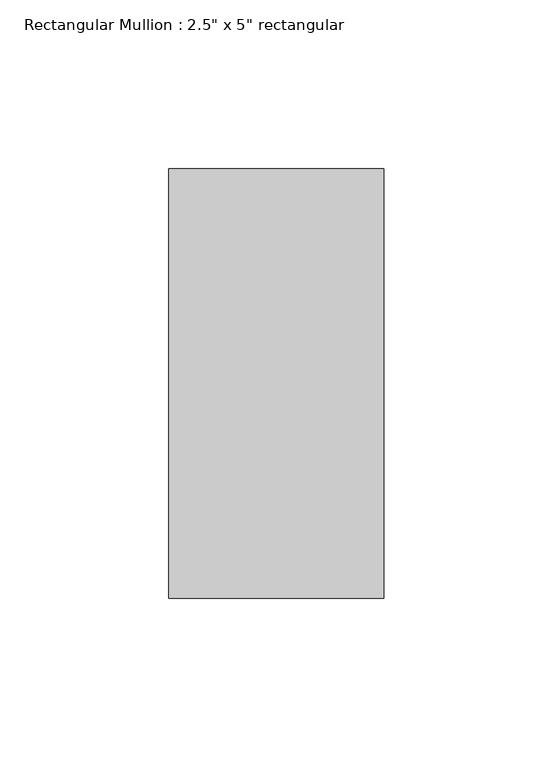
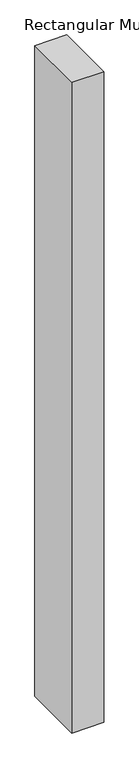
"""IFC4 building model written with IfcOpenShell, lengths in millimetres: member geometry."""

from ifc_helpers import new_model, si_unit, frame, origin, place, context, project, spatial, polyline, outline, extrude, source, transform, mapped, element, save


def member_80f955c2(model_context):
    return source(origin(), model_context, "Body", "SweptSolid", [
        extrude(outline(polyline([(0.0, 63.5), (0.0, -63.5), (-63.5, -63.5), (-63.5, 63.5), (0.0, 63.5)])), frame((0.0, 0.0, -1366.313455), z_axis=(0.0, 0.0, 1.0), x_axis=(1.0, 0.0, 0.0)), (0.0, 0.0, 1.0), 1366.313455),
    ])


if __name__ == "__main__":
    model = new_model("IFC4")
    model_context = context("Model", 3, world=origin())
    ifc_project = project(units=[si_unit("LENGTHUNIT", "METRE", prefix="MILLI")], contexts=[model_context])
    site = spatial("IfcSite", under=ifc_project)
    building = spatial("IfcBuilding", under=site)
    placement = place(None, origin())
    member_shape = member_80f955c2(model_context)
    element("IfcMember", 1, ObjectType="Rectangular Mullion : 2.5\" x 5\" rectangular", at=placement, inside=building, context=model_context, shape_type="MappedRepresentation", body=[
        mapped(member_shape, transform((0.0, 0.0, 0.0), x_axis=(1.0, 0.0, 0.0), y_axis=(0.0, 1.0, 0.0), z_axis=(0.0, 0.0, 1.0))),
    ])
    save(model, "model.ifc")

# Revit data of these elements
# Type "Rectangular Mullion : 2.5\" x 5\" rectangular"
#   built-in parameter 1007304 = 0.416667 (stored number, unit not read)
#   built-in parameter 1007301 = 0.104167 (stored number, unit not read)
#   built-in parameter 1007300 = 0.104167 (stored number, unit not read)
# Element 1 (IfcMember, "Rectangular Mullion : 2.5\" x 5\" rectangular")
#   Materials on its faces: "Aluminum"
# Materials
#   "Aluminum": class "Metal", colour RGB 247 247 247, transparency 0, Description = "Aluminum 6061", Cost = 0
